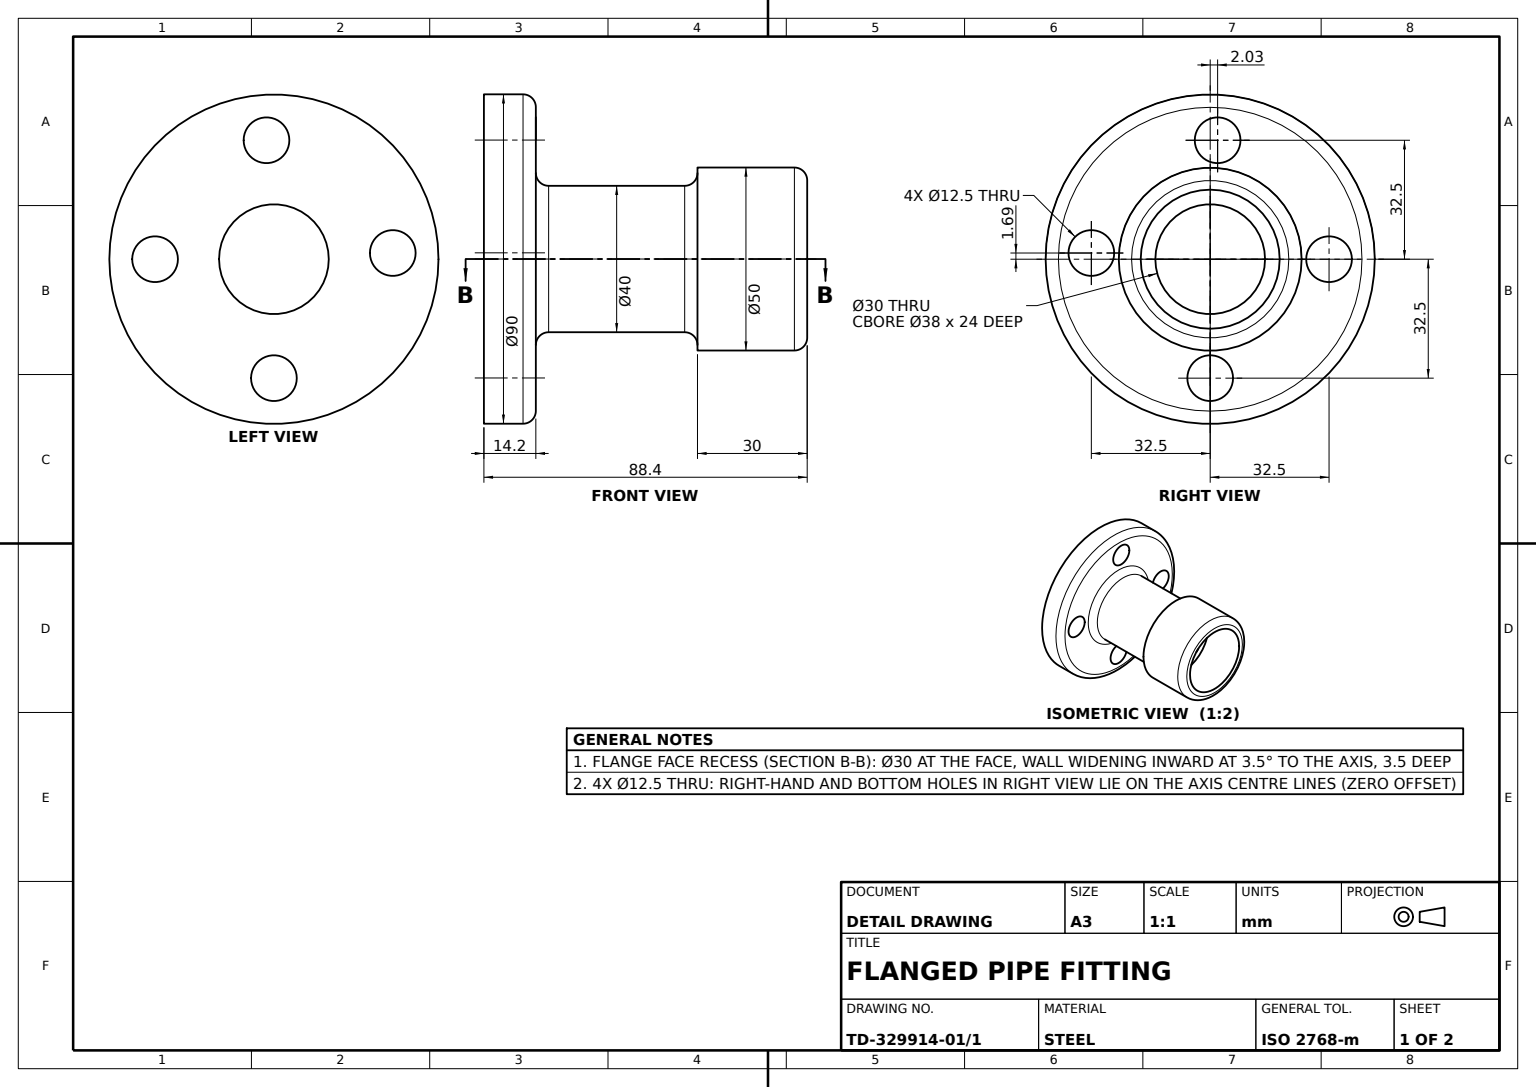
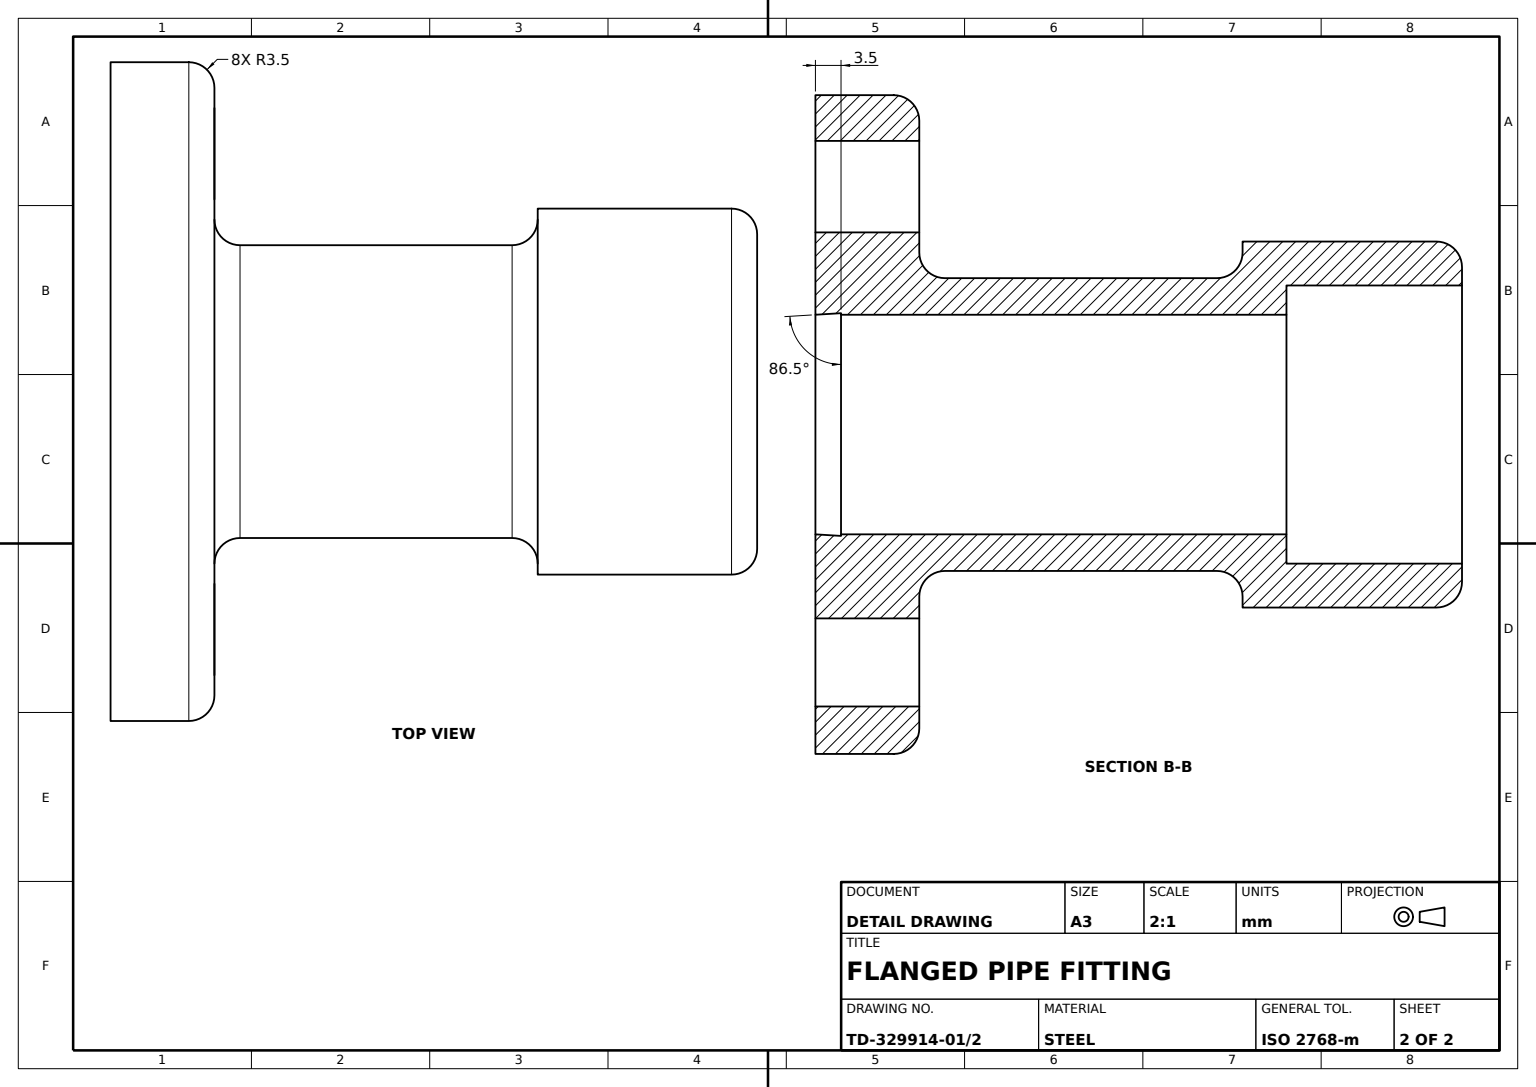
from build123d import *

# Parameters (mm, degrees)
FLANGE_SKETCH_R                = 45
FLANGE_90_DEPTH                = 14.2
NECK_SKETCH_R                  = 20
NECK_40_DEPTH                  = 44.2
HEAD_SKETCH_R                  = 25
HEAD_50_DEPTH                  = 30
BOLT_HOLE_1_SKETCH_R           = 6.25
BOLT_HOLE_1_12_5_DEPTH         = 30
BOLT_HOLE_2_SKETCH_R           = 6.25
BOLT_HOLE_2_12_5_DEPTH         = 30
BOLT_HOLE_3_SKETCH_R           = 6.25
BOLT_HOLE_3_12_5_DEPTH         = 30
BOLT_HOLE_4_SKETCH_R           = 6.25
BOLT_HOLE_4_12_5_DEPTH         = 30
COUNTERBORE_SKETCH_R           = 19
COUNTERBORE_38_DEPTH           = 12
BORE_STEP_SKETCH_R             = 19
BORE_STEP_DEPTH_12_DEPTH       = 12
INNER_BORE_SKETCH_R            = 15
INNER_BORE_30_DEPTH            = 6
NECK_BORE_SKETCH_R             = 15
NECK_BORE_DEPTH                = 44.2
BOTTOM_RECESS_SKETCH_R         = 15
BOTTOM_RECESS_30_DRAFTED_DEPTH = 3.5
BOTTOM_RECESS_30_DRAFTED_DRAFT = 3.5
THROUGH_BORE_SKETCH_R          = 15
THROUGH_BORE_DEPTH             = 80.5
FLANGE_NECK_FILLET_R3_5_R      = 3.5
HEAD_EDGE_FILLET_R3_5_R        = 3.5
NECK_HEAD_FILLET_R3_5_R        = 3.5
FLANGE_EDGE_FILLET_R3_5_R      = 3.5


with BuildPart() as part:
    # Flange Sketch → Flange Ø90 (new body)
    with BuildSketch(Plane(origin=(0, 0, 0), x_dir=(1, 0, 0), z_dir=(0, 1, 0))):
        with Locations(Location((0, 0, 0), (0, 0, 270))):
            Circle(FLANGE_SKETCH_R)
    extrude(amount=FLANGE_90_DEPTH)

    # Neck Sketch → Neck Ø40 (add)
    with BuildSketch(Plane(origin=(0, 14.2, 0), x_dir=(1, 0, 0), z_dir=(0, 1, 0))):
        with Locations(Location((0, 0, 0), (0, 0, 270))):
            Circle(NECK_SKETCH_R)
    extrude(amount=NECK_40_DEPTH)

    # Head Sketch → Head Ø50 (add)
    with BuildSketch(Plane(origin=(0, 58.4, 0), x_dir=(1, 0, 0), z_dir=(0, 1, 0))):
        with Locations(Location((0, 0, 0), (0, 0, 270))):
            Circle(HEAD_SKETCH_R)
    extrude(amount=HEAD_50_DEPTH)

    # Bolt Hole 1 Sketch → Bolt Hole 1 Ø12.5 (cut)
    with BuildSketch(Plane(origin=(0, 14.2, 0), x_dir=(1, 0, 0), z_dir=(0, 1, 0))):
        with Locations(Location((0, 32.5, 0), (0, 0, 270))):
            Circle(BOLT_HOLE_1_SKETCH_R)
    extrude(amount=-BOLT_HOLE_1_12_5_DEPTH, mode=Mode.SUBTRACT)

    # Bolt Hole 2 Sketch → Bolt Hole 2 Ø12.5 (cut)
    with BuildSketch(Plane(origin=(0, 14.2, 0), x_dir=(1, 0, 0), z_dir=(0, 1, 0))):
        with Locations(Location((32.5, 0, 0), (0, 0, 270))):
            Circle(BOLT_HOLE_2_SKETCH_R)
    extrude(amount=-BOLT_HOLE_2_12_5_DEPTH, mode=Mode.SUBTRACT)

    # Bolt Hole 3 Sketch → Bolt Hole 3 Ø12.5 (cut)
    with BuildSketch(Plane(origin=(0, 14.2, 0), x_dir=(1, 0, 0), z_dir=(0, 1, 0))):
        with Locations(Location((-32.5, 2.030932752, 0), (0, 0, 270))):
            Circle(BOLT_HOLE_3_SKETCH_R)
    extrude(amount=-BOLT_HOLE_3_12_5_DEPTH, mode=Mode.SUBTRACT)

    # Bolt Hole 4 Sketch → Bolt Hole 4 Ø12.5 (cut)
    with BuildSketch(Plane(origin=(0, 14.2, 0), x_dir=(1, 0, 0), z_dir=(0, 1, 0))):
        with Locations(Location((-1.69244396, -32.5, 0), (0, 0, 270))):
            Circle(BOLT_HOLE_4_SKETCH_R)
    extrude(amount=-BOLT_HOLE_4_12_5_DEPTH, mode=Mode.SUBTRACT)

    # Counterbore Sketch → Counterbore Ø38 (cut)
    with BuildSketch(Plane(origin=(0, 88.4, 0), x_dir=(1, 0, 0), z_dir=(0, 1, 0))):
        with Locations(Location((0, 0, 0), (0, 0, 270))):
            Circle(COUNTERBORE_SKETCH_R)
    extrude(amount=-COUNTERBORE_38_DEPTH, mode=Mode.SUBTRACT)

    # Bore Step Sketch → Bore Step Depth 12 (cut)
    with BuildSketch(Plane(origin=(0, 76.4, 0), x_dir=(1, 0, 0), z_dir=(0, 1, 0))):
        with Locations(Location((0, 0, 0), (0, 0, 270))):
            Circle(BORE_STEP_SKETCH_R)
    extrude(amount=-BORE_STEP_DEPTH_12_DEPTH, mode=Mode.SUBTRACT)

    # Inner Bore Sketch → Inner Bore Ø30 (cut)
    with BuildSketch(Plane(origin=(0, 64.4, 0), x_dir=(1, 0, 0), z_dir=(0, 1, 0))):
        with Locations(Location((0, 0, 0), (0, 0, 270))):
            Circle(INNER_BORE_SKETCH_R)
    extrude(amount=-INNER_BORE_30_DEPTH, mode=Mode.SUBTRACT)

    # Neck Bore Sketch → Neck Bore (cut)
    with BuildSketch(Plane(origin=(0, 58.4, 0), x_dir=(1, 0, 0), z_dir=(0, 1, 0))):
        with Locations(Location((0, 0, 0), (0, 0, 270))):
            Circle(NECK_BORE_SKETCH_R)
    extrude(amount=-NECK_BORE_DEPTH, mode=Mode.SUBTRACT)


with BuildPart() as bottom_recess_30_drafted_tool:
    # Bottom Recess Sketch → Bottom Recess Ø30 Drafted (with draft: the straight prism first)
    with BuildSketch(Plane.XZ):
        with Locations(Location((0, 0, 0), (0, 0, 90))):
            Circle(BOTTOM_RECESS_SKETCH_R)
    extrude(amount=-BOTTOM_RECESS_30_DRAFTED_DEPTH)
    # Bottom Recess Ø30 Drafted: the draft: its side faces are tilted about the plane it starts from
    bottom_recess_30_drafted_sides = [bottom_recess_30_drafted_tool.faces().sort_by_distance(p)[0] for p in [
        (0, 1.75, -15),
    ]]
    draft(bottom_recess_30_drafted_sides, Plane.XZ, BOTTOM_RECESS_30_DRAFTED_DRAFT)


with BuildPart() as part_1:
    add(part.part)

    # Bottom Recess Ø30 Drafted: cut by bottom_recess_30_drafted_tool
    add(bottom_recess_30_drafted_tool.part, mode=Mode.SUBTRACT)

    # Through Bore Sketch → Through Bore (cut)
    with BuildSketch(Plane(origin=(0, 14.2, 0), x_dir=(1, 0, 0), z_dir=(0, 1, 0))):
        with Locations(Location((0, 0, 0), (0, 0, 270))):
            Circle(THROUGH_BORE_SKETCH_R)
    extrude(amount=-THROUGH_BORE_DEPTH, mode=Mode.SUBTRACT)

    # Flange-Neck Fillet R3.5
    flange_neck_fillet_r3_5_edges = [part_1.edges().sort_by_distance(p)[0] for p in [
        (0, 14.2, -20),
    ]]
    fillet(flange_neck_fillet_r3_5_edges, radius=FLANGE_NECK_FILLET_R3_5_R)

    # Head Edge Fillet R3.5
    head_edge_fillet_r3_5_edges = [part_1.edges().sort_by_distance(p)[0] for p in [
        (0, 88.4, -25),
    ]]
    fillet(head_edge_fillet_r3_5_edges, radius=HEAD_EDGE_FILLET_R3_5_R)

    # Neck-Head Fillet R3.5
    neck_head_fillet_r3_5_edges = [part_1.edges().sort_by_distance(p)[0] for p in [
        (0, 58.4, -20),
    ]]
    fillet(neck_head_fillet_r3_5_edges, radius=NECK_HEAD_FILLET_R3_5_R)

    # Flange Edge Fillet R3.5
    flange_edge_fillet_r3_5_edges = [part_1.edges().sort_by_distance(p)[0] for p in [
        (0, 14.2, -45),
    ]]
    fillet(flange_edge_fillet_r3_5_edges, radius=FLANGE_EDGE_FILLET_R3_5_R)


solid = part_1.part
